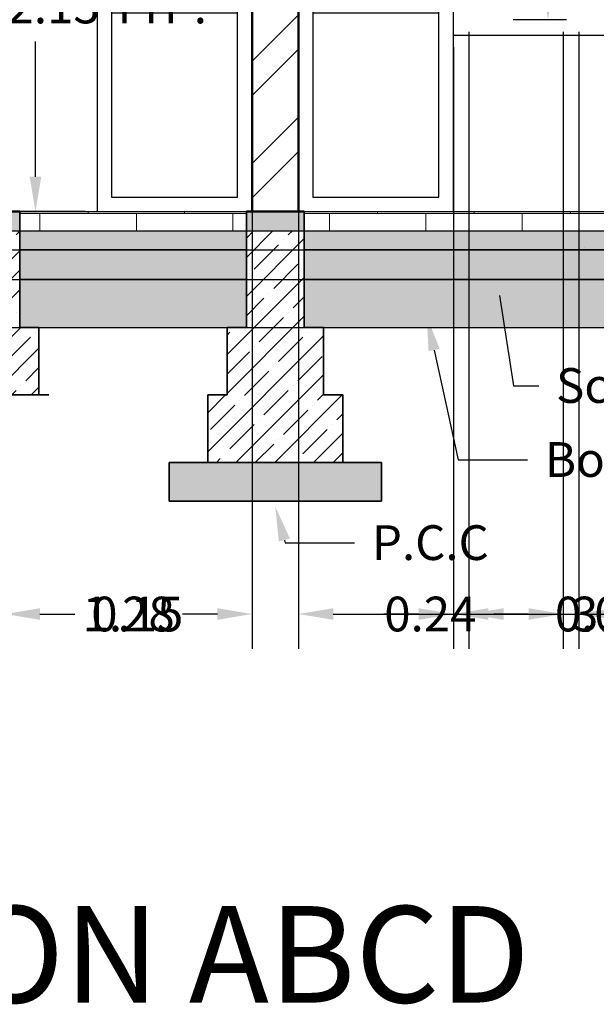
# Model space of a CAD drawing. Units: metres. Extents: x 22.1 to 34.4, y 4.4 to 12.4.
# Tile 2 of 8: x 26.6 to 29.6, y 4.4 to 9.5. Entities that reach past the tile are written whole.
import ezdxf
from ezdxf import colors
from ezdxf.entities.mleader import LeaderData, LeaderLine
from ezdxf.math import Vec2, Vec3

# ---------------------------------------------------------------- set-up
doc = ezdxf.new("R2010")
doc.units = ezdxf.units.M
doc.header["$MEASUREMENT"] = 0
for name, color, linetype, lineweight in [('A-ANNO-DIMS', 2, 'Continuous', 18), ('A-ANNO-TEXT', 7, 'Continuous', 18), ('A-DOOR', 4, 'Continuous', 25), ('A-FLOR', 3, 'Continuous', 25), ('A-FLOR-PATT', 252, 'Continuous', 13), ('A-GLAZ', 4, 'Continuous', 25), ('A-WALL', 7, 'Continuous', 50), ('A-WALL-PATT', 8, 'Continuous', 18), ('S-FNDN', 1, 'Continuous', 35), ('S-FNDN-PATT', 8, 'Continuous', 13), ('S-SLAB-PATT', 8, 'Continuous', 13)]:
    doc.layers.add(name, color=color, linetype=linetype, lineweight=lineweight)
doc.styles.get("Standard").update_dxf_attribs({"font": 'arial.ttf'})
doc.dimstyles.get("Standard").update_dxf_attribs({"dimtxt": 0.18, "dimasz": 0.18, "dimexe": 0.18, "dimexo": 0.0625, "dimgap": 0.09, "dimtad": 0, "dimtih": 1, "dimtoh": 1, "dimzin": 0, "dimdsep": 46, "dimtxsty": 'Standard', "dimcen": 0.09, "dimadec": 0, "dimazin": 0, "dimtfac": 1, "dimtofl": 0, "dimtmove": 0, "dimatfit": 3, "dimfxl": 1, "dimtolj": 1, "dimtzin": 0, "dimarcsym": 0})

# ---------------------------------------------------------------- blocks, each defined once
blk = doc.blocks.new('DOOR-800')
for p, q in [((26.4206, 10.6399), (25.6173, 10.6399)), ((25.6173, 10.6399), (25.6173, 8.5099)), ((26.4206, 8.5099), (26.4206, 10.6399)), ((25.6923, 10.5649), (25.6923, 8.5849)), ((26.3456, 10.5649), (25.6923, 10.5649)), ((26.3456, 8.5849), (26.3456, 10.5649)), ((25.6923, 9.6099), (26.3456, 9.6099)), ((25.6923, 9.5399), (26.3456, 9.5399)), ((25.6923, 8.5849), (26.3456, 8.5849)), ((25.6173, 8.5099), (26.4206, 8.5099))]:
    blk.add_line(p, q)
blk = doc.blocks.new('*D16')
at = {"layer": 'A-ANNO-DIMS', "color": 0, "lineweight": -2, "transparency": 16777216}
for p, q in [((26.9843, 10.6399), (26.5473, 10.6399)), ((26.7273, 10.4599), (26.7273, 9.7581)), ((26.7273, 8.6899), (26.7273, 9.3917)), ((26.9843, 8.5099), (26.5473, 8.5099))]:
    blk.add_line(p, q, dxfattribs=at)
at = {"layer": 'A-ANNO-DIMS', "color": 0, "transparency": 16777216}
for points in [[(26.6973, 10.4599), (26.7573, 10.4599), (26.7273, 10.6399)], [(26.6973, 8.6899), (26.7573, 8.6899), (26.7273, 8.5099)]]:
    blk.add_solid(points, dxfattribs=at)
at = {"layer": 'Defpoints', "color": 0, "transparency": 16777216}
for p in [(26.7273, 10.6399), (27.0468, 10.6399), (27.0468, 8.5099)]:
    blk.add_point(p, dxfattribs=at)
at = {"layer": 'A-ANNO-DIMS', "color": 0, "transparency": 16777216, "insert": (26.7273, 9.5749), "char_height": 0.18, "attachment_point": 5}
blk.add_mtext('\\A1;DOOR 2.13 TYP.', dxfattribs=at)
blk = doc.blocks.new('*D20')
at = {"layer": 'A-ANNO-DIMS', "color": 0, "lineweight": -2, "transparency": 16777216}
for p, q in [((29.4798, 10.5649), (29.2032, 10.5649)), ((29.3832, 10.3849), (29.3832, 10.2176)), ((29.3832, 9.6839), (29.3832, 9.8512)), ((29.4798, 9.5039), (29.2032, 9.5039))]:
    blk.add_line(p, q, dxfattribs=at)
at = {"layer": 'A-ANNO-DIMS', "color": 0, "transparency": 16777216}
for points in [[(29.3532, 10.3849), (29.4132, 10.3849), (29.3832, 10.5649)], [(29.3532, 9.6839), (29.4132, 9.6839), (29.3832, 9.5039)]]:
    blk.add_solid(points, dxfattribs=at)
at = {"layer": 'Defpoints', "color": 0, "transparency": 16777216}
for p in [(29.3832, 10.5649), (29.5423, 10.5649), (29.5423, 9.5039)]:
    blk.add_point(p, dxfattribs=at)
at = {"layer": 'A-ANNO-DIMS', "color": 0, "transparency": 16777216, "insert": (29.3832, 10.0344), "char_height": 0.18, "attachment_point": 5}
blk.add_mtext('\\A1;WINDOW PANE 530 1.06 TYP.', dxfattribs=at)
blk = doc.blocks.new('*D23')
at = {"layer": 'A-ANNO-DIMS', "color": 0, "lineweight": -2, "transparency": 16777216}
for p, q in [((28.0901, 11.4474), (28.0901, 6.2449)), ((31.5381, 11.4474), (31.5381, 6.2449)), ((28.2701, 6.4249), (29.4202, 6.4249)), ((31.3581, 6.4249), (30.2079, 6.4249))]:
    blk.add_line(p, q, dxfattribs=at)
at = {"layer": 'A-ANNO-DIMS', "color": 0, "transparency": 16777216}
for points in [[(28.2701, 6.4549), (28.2701, 6.3949), (28.0901, 6.4249)], [(31.3581, 6.4549), (31.3581, 6.3949), (31.5381, 6.4249)]]:
    blk.add_solid(points, dxfattribs=at)
at = {"layer": 'Defpoints', "color": 0, "transparency": 16777216}
for p in [(28.0901, 11.5099), (31.5381, 11.5099), (31.5381, 6.4249)]:
    blk.add_point(p, dxfattribs=at)
at = {"layer": 'A-ANNO-DIMS', "color": 0, "transparency": 16777216, "insert": (29.8141, 6.4249), "char_height": 0.18, "attachment_point": 5}
blk.add_mtext('\\A1;3.448', dxfattribs=at)
blk = doc.blocks.new('*D26')
at = {"layer": 'A-ANNO-DIMS', "color": 0, "lineweight": -2, "transparency": 16777216}
for p, q in [((27.8501, 11.4474), (27.8501, 6.2449)), ((28.0901, 11.4474), (28.0901, 6.2449)), ((27.6701, 6.4249), (27.4901, 6.4249)), ((28.2701, 6.4249), (28.4501, 6.4249))]:
    blk.add_line(p, q, dxfattribs=at)
at = {"layer": 'A-ANNO-DIMS', "color": 0, "transparency": 16777216}
for points in [[(27.6701, 6.4549), (27.6701, 6.3949), (27.8501, 6.4249)], [(28.2701, 6.4549), (28.2701, 6.3949), (28.0901, 6.4249)]]:
    blk.add_solid(points, dxfattribs=at)
at = {"layer": 'Defpoints', "color": 0, "transparency": 16777216}
for p in [(27.8501, 11.5099), (28.0901, 11.5099), (28.0901, 6.4249)]:
    blk.add_point(p, dxfattribs=at)
at = {"layer": 'A-ANNO-DIMS', "color": 0, "transparency": 16777216, "insert": (28.7735, 6.4249), "char_height": 0.18, "attachment_point": 5}
blk.add_mtext('\\A1;0.24', dxfattribs=at)
blk = doc.blocks.new('*D31')
at = {"layer": 'A-ANNO-DIMS', "color": 0, "lineweight": -2, "transparency": 16777216}
for p, q in [((26.4206, 8.4474), (26.4206, 6.2449)), ((26.5706, 8.4474), (26.5706, 6.2449)), ((26.2406, 6.4249), (26.0606, 6.4249)), ((26.7506, 6.4249), (26.9306, 6.4249))]:
    blk.add_line(p, q, dxfattribs=at)
at = {"layer": 'A-ANNO-DIMS', "color": 0, "transparency": 16777216}
for points in [[(26.2406, 6.4549), (26.2406, 6.3949), (26.4206, 6.4249)], [(26.7506, 6.4549), (26.7506, 6.3949), (26.5706, 6.4249)]]:
    blk.add_solid(points, dxfattribs=at)
at = {"layer": 'Defpoints', "color": 0, "transparency": 16777216}
for p in [(26.4206, 8.5099), (26.5706, 8.5099), (26.5706, 6.4249)]:
    blk.add_point(p, dxfattribs=at)
at = {"layer": 'A-ANNO-DIMS', "color": 0, "transparency": 16777216, "insert": (27.255, 6.4249), "char_height": 0.18, "attachment_point": 5}
blk.add_mtext('\\A1;0.15', dxfattribs=at)
blk = doc.blocks.new('*D32')
at = {"layer": 'A-ANNO-DIMS', "color": 0, "lineweight": -2, "transparency": 16777216}
for p, q in [((26.5706, 8.4474), (26.5706, 6.2449)), ((27.8501, 8.4474), (27.8501, 6.2449)), ((26.7506, 6.4249), (26.8948, 6.4249)), ((27.6701, 6.4249), (27.5258, 6.4249))]:
    blk.add_line(p, q, dxfattribs=at)
at = {"layer": 'A-ANNO-DIMS', "color": 0, "transparency": 16777216}
for points in [[(26.7506, 6.4549), (26.7506, 6.3949), (26.5706, 6.4249)], [(27.6701, 6.4549), (27.6701, 6.3949), (27.8501, 6.4249)]]:
    blk.add_solid(points, dxfattribs=at)
at = {"layer": 'Defpoints', "color": 0, "transparency": 16777216}
for p in [(26.5706, 8.5099), (27.8501, 8.5099), (27.8501, 6.4249)]:
    blk.add_point(p, dxfattribs=at)
at = {"layer": 'A-ANNO-DIMS', "color": 0, "transparency": 16777216, "insert": (27.2103, 6.4249), "char_height": 0.18, "attachment_point": 5}
blk.add_mtext('\\A1;1.28', dxfattribs=at)
blk = doc.blocks.new('*D34')
at = {"layer": 'A-ANNO-DIMS', "color": 0, "lineweight": -2, "transparency": 16777216}
for p, q in [((28.8933, 9.3614), (28.8933, 6.2449)), ((31.3293, 9.3614), (31.3293, 6.2449)), ((29.0733, 6.4249), (29.7162, 6.4249)), ((31.1493, 6.4249), (30.5065, 6.4249))]:
    blk.add_line(p, q, dxfattribs=at)
at = {"layer": 'A-ANNO-DIMS', "color": 0, "transparency": 16777216}
for points in [[(29.0733, 6.4549), (29.0733, 6.3949), (28.8933, 6.4249)], [(31.1493, 6.4549), (31.1493, 6.3949), (31.3293, 6.4249)]]:
    blk.add_solid(points, dxfattribs=at)
at = {"layer": 'Defpoints', "color": 0, "transparency": 16777216}
for p in [(28.8933, 9.4239), (31.3293, 9.4239), (31.3293, 6.4249)]:
    blk.add_point(p, dxfattribs=at)
at = {"layer": 'A-ANNO-DIMS', "color": 0, "transparency": 16777216, "insert": (30.1113, 6.4249), "char_height": 0.18, "attachment_point": 5}
blk.add_mtext('\\A1;2.436', dxfattribs=at)
blk = doc.blocks.new('*D35')
at = {"layer": 'A-ANNO-DIMS', "color": 0, "lineweight": -2, "transparency": 16777216}
for p, q in [((28.9733, 9.4414), (28.9733, 6.2449)), ((28.8933, 9.3614), (28.8933, 6.2449)), ((28.7133, 6.4249), (28.5333, 6.4249)), ((29.1533, 6.4249), (29.3333, 6.4249))]:
    blk.add_line(p, q, dxfattribs=at)
at = {"layer": 'A-ANNO-DIMS', "color": 0, "transparency": 16777216}
for points in [[(28.7133, 6.4549), (28.7133, 6.3949), (28.8933, 6.4249)], [(29.1533, 6.4549), (29.1533, 6.3949), (28.9733, 6.4249)]]:
    blk.add_solid(points, dxfattribs=at)
at = {"layer": 'Defpoints', "color": 0, "transparency": 16777216}
for p in [(28.9733, 9.5039), (28.8933, 9.4239), (28.9733, 6.4249)]:
    blk.add_point(p, dxfattribs=at)
at = {"layer": 'A-ANNO-DIMS', "color": 0, "transparency": 16777216, "insert": (29.6573, 6.4249), "char_height": 0.18, "attachment_point": 5}
blk.add_mtext('\\A1;0.08', dxfattribs=at)
blk = doc.blocks.new('*D36')
at = {"layer": 'A-ANNO-DIMS', "color": 0, "lineweight": -2, "transparency": 16777216}
for p, q in [((29.4623, 9.4414), (29.4623, 6.2449)), ((29.5423, 9.4414), (29.5423, 6.2449)), ((29.2823, 6.4249), (29.1023, 6.4249)), ((29.7223, 6.4249), (29.9023, 6.4249))]:
    blk.add_line(p, q, dxfattribs=at)
at = {"layer": 'A-ANNO-DIMS', "color": 0, "transparency": 16777216}
for points in [[(29.2823, 6.4549), (29.2823, 6.3949), (29.4623, 6.4249)], [(29.7223, 6.4549), (29.7223, 6.3949), (29.5423, 6.4249)]]:
    blk.add_solid(points, dxfattribs=at)
at = {"layer": 'Defpoints', "color": 0, "transparency": 16777216}
for p in [(29.4623, 9.5039), (29.5423, 9.5039), (29.5423, 6.4249)]:
    blk.add_point(p, dxfattribs=at)
at = {"layer": 'A-ANNO-DIMS', "color": 0, "transparency": 16777216, "insert": (30.2263, 6.4249), "char_height": 0.18, "attachment_point": 5}
blk.add_mtext('\\A1;0.08', dxfattribs=at)
blk = doc.blocks.new('*D44')
at = {"layer": 'A-ANNO-DIMS', "color": 0, "lineweight": -2, "transparency": 16777216}
for p, q in [((33.6737, 8.6899), (33.6737, 8.8699)), ((24.8474, 8.5099), (33.8537, 8.5099)), ((24.5474, 8.4099), (33.8537, 8.4099)), ((33.6737, 8.2299), (33.6737, 8.0499)), ((33.6737, 8.0499), (33.4937, 8.0499))]:
    blk.add_line(p, q, dxfattribs=at)
at = {"layer": 'A-ANNO-DIMS', "color": 0, "transparency": 16777216}
for points in [[(33.6437, 8.6899), (33.7037, 8.6899), (33.6737, 8.5099)], [(33.6437, 8.2299), (33.7037, 8.2299), (33.6737, 8.4099)]]:
    blk.add_solid(points, dxfattribs=at)
at = {"layer": 'Defpoints', "color": 0, "transparency": 16777216}
for p in [(24.7849, 8.5099), (24.4849, 8.4099), (33.6737, 8.4099)]:
    blk.add_point(p, dxfattribs=at)
at = {"layer": 'A-ANNO-DIMS', "color": 0, "transparency": 16777216, "insert": (33.1702, 8.0499), "char_height": 0.18, "attachment_point": 5}
blk.add_mtext('\\A1;0.10', dxfattribs=at)
blk = doc.blocks.new('*D45')
at = {"layer": 'A-ANNO-DIMS', "color": 0, "lineweight": -2, "transparency": 16777216}
for p, q in [((33.6737, 8.5899), (33.6737, 8.7699)), ((24.5474, 8.4099), (33.8537, 8.4099)), ((24.8474, 8.3119), (33.8537, 8.3119)), ((33.6737, 8.1319), (33.6737, 7.9519)), ((33.6737, 7.9519), (33.4937, 7.9519))]:
    blk.add_line(p, q, dxfattribs=at)
at = {"layer": 'A-ANNO-DIMS', "color": 0, "transparency": 16777216}
for points in [[(33.6437, 8.5899), (33.7037, 8.5899), (33.6737, 8.4099)], [(33.6437, 8.1319), (33.7037, 8.1319), (33.6737, 8.3119)]]:
    blk.add_solid(points, dxfattribs=at)
at = {"layer": 'Defpoints', "color": 0, "transparency": 16777216}
for p in [(24.4849, 8.4099), (24.7849, 8.3119), (33.6737, 8.3119)]:
    blk.add_point(p, dxfattribs=at)
at = {"layer": 'A-ANNO-DIMS', "color": 0, "transparency": 16777216, "insert": (33.0998, 7.9519), "char_height": 0.18, "attachment_point": 5}
blk.add_mtext('\\A1;0.098', dxfattribs=at)
blk = doc.blocks.new('*D46')
at = {"layer": 'A-ANNO-DIMS', "color": 0, "lineweight": -2, "transparency": 16777216}
for p, q in [((33.6737, 8.4919), (33.6737, 8.6719)), ((24.8474, 8.3119), (33.8537, 8.3119)), ((24.8474, 8.1578), (33.8537, 8.1578)), ((33.6737, 7.9778), (33.6737, 7.7978)), ((33.6737, 7.7978), (33.4937, 7.7978))]:
    blk.add_line(p, q, dxfattribs=at)
at = {"layer": 'A-ANNO-DIMS', "color": 0, "transparency": 16777216}
for points in [[(33.6437, 8.4919), (33.7037, 8.4919), (33.6737, 8.3119)], [(33.6437, 7.9778), (33.7037, 7.9778), (33.6737, 8.1578)]]:
    blk.add_solid(points, dxfattribs=at)
at = {"layer": 'Defpoints', "color": 0, "transparency": 16777216}
for p in [(24.7849, 8.3119), (24.7849, 8.1578), (33.6737, 8.1578)]:
    blk.add_point(p, dxfattribs=at)
at = {"layer": 'A-ANNO-DIMS', "color": 0, "transparency": 16777216, "insert": (33.1692, 7.7978), "char_height": 0.18, "attachment_point": 5}
blk.add_mtext('\\A1;0.15', dxfattribs=at)
blk = doc.blocks.new('*D47')
at = {"layer": 'A-ANNO-DIMS', "color": 0, "lineweight": -2, "transparency": 16777216}
for p, q in [((33.6737, 8.3378), (33.6737, 8.5178)), ((24.8474, 8.1578), (33.8537, 8.1578)), ((24.8474, 7.9099), (33.8537, 7.9099)), ((33.6737, 7.7299), (33.6737, 7.5499)), ((33.6737, 7.5499), (33.4937, 7.5499))]:
    blk.add_line(p, q, dxfattribs=at)
at = {"layer": 'A-ANNO-DIMS', "color": 0, "transparency": 16777216}
for points in [[(33.6437, 8.3378), (33.7037, 8.3378), (33.6737, 8.1578)], [(33.6437, 7.7299), (33.7037, 7.7299), (33.6737, 7.9099)]]:
    blk.add_solid(points, dxfattribs=at)
at = {"layer": 'Defpoints', "color": 0, "transparency": 16777216}
for p in [(24.7849, 8.1578), (24.7849, 7.9099), (33.6737, 7.9099)]:
    blk.add_point(p, dxfattribs=at)
at = {"layer": 'A-ANNO-DIMS', "color": 0, "transparency": 16777216, "insert": (33.1692, 7.5499), "char_height": 0.18, "attachment_point": 5}
blk.add_mtext('\\A1;0.25', dxfattribs=at)

msp = doc.modelspace()

# ---------------------------------------------------------------- hatches: boundary and pattern name
at = {"layer": 'A-FLOR-PATT'}
h = msp.add_hatch(dxfattribs=at)
h.set_pattern_fill('BRICK', color=256)
h.paths.add_polyline_path([(31.5081, 8.5099), (28.1201, 8.5099), (28.1201, 8.4099), (31.5081, 8.4099)])
h.paths.add_polyline_path([(27.8201, 8.5099), (27.0468, 8.5099), (26.6456, 8.5099), (26.6456, 8.4099), (27.8201, 8.4099)])
h.paths.add_polyline_path([(26.3456, 8.5099), (25.6173, 8.5099), (24.7849, 8.5099), (24.7849, 8.4099), (26.3456, 8.4099)])
h = msp.add_hatch(dxfattribs=at)
h.set_pattern_fill('AR-SAND', color=256, scale=0.57)
h.paths.add_polyline_path([(26.3456, 8.4099), (24.7849, 8.4099), (24.7849, 8.3119), (26.3456, 8.3119)])
h.paths.add_polyline_path([(27.8201, 8.4099), (26.6456, 8.4099), (26.6456, 8.3119), (27.8201, 8.3119)])
h.paths.add_polyline_path([(31.5081, 8.4099), (28.1201, 8.4099), (28.1201, 8.3119), (31.5081, 8.3119)])
h = msp.add_hatch(dxfattribs=at)
h.set_pattern_fill('AR-SAND', color=256, scale=0.57)
h.paths.add_polyline_path([(31.5081, 8.4099), (28.1201, 8.4099), (28.1201, 8.3119), (31.5081, 8.3119)])
h.paths.add_polyline_path([(27.8201, 8.4099), (26.6456, 8.4099), (26.6456, 8.3119), (27.8201, 8.3119)])
h.paths.add_polyline_path([(26.3456, 8.4099), (24.7849, 8.4099), (24.7849, 8.3119), (26.3456, 8.3119)])
h = msp.add_hatch(dxfattribs=at)
h.set_pattern_fill('AR-SAND', color=256, scale=0.04)
h.paths.add_polyline_path([(26.3456, 8.4099), (24.7849, 8.4099), (24.7849, 8.3119), (26.3456, 8.3119)])
h.paths.add_polyline_path([(27.8201, 8.4099), (26.6456, 8.4099), (26.6456, 8.3119), (27.8201, 8.3119)])
h.paths.add_polyline_path([(31.5081, 8.4099), (28.1201, 8.4099), (28.1201, 8.3119), (31.5081, 8.3119)])
h = msp.add_hatch(dxfattribs=at)
h.set_pattern_fill('GRAVEL', color=256, scale=0.18)
h.set_pattern_definition([(228.012788, (0.1296, 0.18), (-1.44, -1.62), [0.0242165, -2.39743585]), (184.96974, (0.1134, 0.162), (2.16, 0.18), [0.0415562, -4.1140665]), (132.510447, (0.072, 0.1584), (1.8, -1.98), [0.0293018, -2.9008859]), (267.27369, (0.0018, 0.1134), (0.18, 3.6), [0.0378428, -3.74644045]), (292.833654, (0, 0.0756), (-0.9, 2.16), [0.0371079, -3.6736872]), (357.27369, (0.0144, 0.0414), (-3.6, 0.18), [0.0378428, -3.74644045]), (37.69424, (0.0522, 0.0396), (-2.34, -1.8), [0.0500452, -4.9544727]), (72.255328, (0.0918, 0.0702), (1.26, 3.96), [0.0472478, -4.6775379]), (121.429566, (0.1062, 0.1152), (-1.44, 2.34), [0.037971, -3.7591332]), (175.23636, (0.0864, 0.1476), (1.98, -0.18), [0.0433498, -2.1241373]), (222.397438, (0.0432, 0.1512), (-2.16, -1.98), [0.0560606, -5.5500075]), (138.814075, (0.18, 0.1116), (-1.26, 1.08), [0.0191342, -1.8942921]), (171.469234, (0.1656, 0.1242), (2.34, -0.36), [0.0364027, -3.60387205]), (225, (0.1296, 0.1296), (0, -0.18), [0.0254558, -0.2291027]), (203.19859, (0.117, 0.1512), (0.9, 0.36), [0.0137084, -1.3571307]), (291.80141, (0.1044, 0.1458), (-0.18, 0.54), [0.0193865, -0.9499431]), (30.96376, (0.1116, 0.1278), (0.54, 0.36), [0.0314872, -1.0180841]), (161.56505, (0.1386, 0.144), (0.36, -0.18), [0.0227684, -0.5464416]), (16.38954, (0, 0.1458), (1.8, 0.54), [0.031896, -3.1577121]), (70.346176, (0.0306, 0.1548), (-0.72, -1.98), [0.026759, -2.6491334]), (293.19859, (0.1386, 0.18), (-0.36, 0.9), [0.0274167, -1.3434225]), (343.61046, (0.1494, 0.1548), (-1.8, 0.54), [0.031896, -3.1577121]), (339.443955, (0, 0.0342), (-0.9, 0.36), [0.0307584, -1.5071623]), (294.77514, (0.0288, 0.0234), (-0.9, 1.98), [0.025772, -2.55143575]), (66.80141, (0.1404, 0), (0.36, 0.9), [0.0274167, -1.3434225]), (17.354025, (0.1512, 0.0252), (-2.34, -0.72), [0.0301736, -2.98717625]), (69.443955, (0.0522, 0), (-0.36, -0.9), [0.0153792, -1.5225415]), (101.30993, (0.1296, 0), (-0.18, 0.72), [0.0091782, -0.9086453]), (165.96376, (0.1278, 0.009), (0.54, -0.18), [0.0371079, -0.7050511]), (186.009006, (0.0918, 0.018), (1.8, 0.18), [0.034389, -3.4045062]), (303.69007, (0.1116, 0.1116), (-0.18, 0.36), [0.02596, -0.6230393]), (353.157227, (0.126, 0.09), (3.06, -0.36), [0.0453229, -4.4869613]), (60.945396, (0.171, 0.0846), (-0.72, -1.26), [0.0185321, -1.8346813]), (90, (0.18, 0.1008), (-0.18, 0.18), [0.0108, -0.1692]), (120.256437, (0.0882, 0.0234), (0.72, -1.26), [0.0250063, -2.4756336]), (48.012788, (0.0756, 0.045), (1.44, 1.62), [0.048433, -2.3732194]), (0, (0.108, 0.081), (0.18, 0.18), [0.0468, -0.1332]), (325.304846, (0.1548, 0.081), (1.8, -1.26), [0.0284605, -2.8175894]), (254.0546, (0.1782, 0.0648), (-0.18, -0.72), [0.0262084, -1.2842114]), (207.645975, (0.171, 0.0396), (-3.42, -1.8), [0.0426717, -4.22450535]), (175.42608, (0.1332, 0.0198), (-2.34, 0.18), [0.0451438, -4.4692332])])
h.paths.add_polyline_path([(26.3456, 8.1578), (24.7849, 8.1578), (24.7849, 7.9099), (24.8849, 7.9099), (26.3456, 7.9099)])
h.paths.add_polyline_path([(27.8201, 8.1578), (26.6456, 8.1578), (26.6456, 7.9099), (26.7456, 7.9099), (27.8201, 7.9099)])
h.paths.add_polyline_path([(31.5081, 8.1578), (28.1201, 8.1578), (28.1201, 7.9099), (31.4081, 7.9099), (31.5081, 7.9099)])
at = {"layer": 'A-WALL-PATT'}
h = msp.add_hatch(dxfattribs=at)
h.set_pattern_fill('ANSI32', color=256)
h.paths.add_polyline_path([(24.7549, 11.5099), (24.5149, 11.5099), (24.5149, 11.1399), (24.7549, 11.1399)])
h.paths.add_polyline_path([(24.7549, 10.6399), (24.5149, 10.6399), (24.5149, 8.5099), (24.6349, 8.5099), (24.7549, 8.5099)])
h.paths.add_polyline_path([(26.5706, 11.5099), (26.4206, 11.5099), (26.4206, 8.5099), (26.5706, 8.5099)])
h.paths.add_polyline_path([(28.0901, 10.6399), (28.0901, 11.5099), (27.8501, 11.5099), (27.8501, 8.5099), (28.0901, 8.5099)])
h.paths.add_polyline_path([(31.7781, 11.5099), (31.5381, 11.5099), (31.5381, 8.5099), (31.6581, 8.5099), (31.7781, 8.5099)])
at = {"layer": 'S-FNDN-PATT'}
h = msp.add_hatch(dxfattribs=at)
h.set_pattern_fill('ANSI35', color=256, scale=0.57)
h.paths.add_polyline_path([(24.3849, 7.5599), (24.2849, 7.5599), (24.2849, 7.2099), (24.9849, 7.2099), (24.9849, 7.5599), (24.8849, 7.5599), (24.8849, 7.9099), (24.7849, 7.9099), (24.7849, 8.4099), (24.4849, 8.4099), (24.4849, 7.9099), (24.3849, 7.9099)])
h.paths.add_polyline_path([(27.7201, 7.5599), (27.6201, 7.5599), (27.6201, 7.2099), (28.3201, 7.2099), (28.3201, 7.5599), (28.2201, 7.5599), (28.2201, 7.9099), (28.1201, 7.9099), (28.1201, 8.4099), (27.8201, 8.4099), (27.8201, 7.9099), (27.7201, 7.9099)])
h.paths.add_polyline_path([(26.7456, 7.9099), (26.6456, 7.9099), (26.6456, 8.4099), (26.3456, 8.4099), (26.3456, 7.9099), (26.2456, 7.9099), (26.2456, 7.5599), (26.4616, 7.5599), (26.4616, 7.6127), (26.4825, 7.5003), (26.4825, 7.5599), (26.7456, 7.5599)])
h.paths.add_polyline_path([(31.8581, 7.5599), (31.8581, 7.9099), (31.8081, 7.9099), (31.8081, 8.4099), (31.5081, 8.4099), (31.5081, 7.9099), (31.4581, 7.9099), (31.4581, 7.5599), (31.3581, 7.5599), (31.3581, 7.2099), (31.9581, 7.2099), (31.9581, 7.5599)])
at = {"layer": 'S-SLAB-PATT'}
h = msp.add_hatch(dxfattribs=at)
h.set_pattern_fill('AR-CONC', color=256, scale=0.04)
h.set_pattern_definition([(50, (0, 0), (0.286904, -0.0251009), [0.03, -0.33]), (355, (0, 0), (-0.0555005, 0.3008769), [0.024, -0.264]), (100.4514, (0.0239, -0.0021), (0.2314035, 0.275776), [0.025496, -0.2804568]), (46.1842, (0, 0.08), (0.4268965, -0.0662077), [0.045, -0.495]), (96.6356, (0.03557, 0.0745), (0.373865, 0.3896474), [0.038244, -0.4206855]), (351.1842, (0, 0.08), (0.373865, 0.3896474), [0.036, -0.396]), (21, (0.04, 0.06), (0.2387628, -0.1610476), [0.03, -0.33]), (326, (0.04, 0.06), (0.0973261, 0.29006), [0.024, -0.264]), (71.4514, (0.0599, 0.04658), (0.336089, 0.1290125), [0.025496, -0.2804568]), (37.5, (0, 0), (0.00486394, 0.13315754), [0, -0.2608, 0, -0.268, 0, -0.265]), (7.5, (0, 0), (0.1052278, 0.1577647), [0, -0.1528, 0, -0.2548, 0, -0.101]), (327.5, (-0.0892, 0), (0.21352897, -0.00902195), [0, -0.1, 0, -0.312, 0, -0.414]), (317.5, (-0.1292, 0), (0.2332745, 0.040042), [0, -0.13, 0, -0.2072, 0, -0.294])])
h.paths.add_polyline_path([(31.9781, 11.6599), (24.3149, 11.6599), (24.3149, 11.5099), (24.5149, 11.5099), (31.7781, 11.5099), (31.9781, 11.5099)])
h.paths.add_polyline_path([(25.1849, 7.2099), (24.9849, 7.2099), (24.0849, 7.2099), (24.0849, 7.0099), (25.1849, 7.0099)])
h.paths.add_polyline_path([(32.2081, 7.2099), (32.0081, 7.2099), (31.1081, 7.2099), (31.1081, 7.0099), (32.2081, 7.0099)])
h.paths.add_polyline_path([(28.5201, 7.2099), (28.3201, 7.2099), (27.4201, 7.2099), (27.4201, 7.0099), (28.5201, 7.0099)])
h.paths.add_polyline_path([(24.7849, 8.5099), (24.6349, 8.5099), (24.5149, 8.5099), (24.4849, 8.5099), (24.4849, 8.4099), (24.7849, 8.4099)])
h.paths.add_polyline_path([(26.6456, 8.5099), (26.3456, 8.5099), (26.3456, 8.4099), (26.6456, 8.4099)])
h.paths.add_polyline_path([(28.1201, 8.5099), (28.0901, 8.5099), (27.8201, 8.5099), (27.8201, 8.4099), (28.1201, 8.4099)])
h.paths.add_polyline_path([(31.8081, 8.5099), (31.6581, 8.5099), (31.5381, 8.5099), (31.5081, 8.5099), (31.5081, 8.4099), (31.8081, 8.4099)])
h.paths.add_polyline_path([(26.3456, 8.3119), (24.7849, 8.3119), (24.7849, 8.1578), (26.3456, 8.1578)])
h.paths.add_polyline_path([(27.8201, 8.3119), (26.6456, 8.3119), (26.6456, 8.1578), (27.8201, 8.1578)])
h.paths.add_polyline_path([(31.5081, 8.3119), (28.1201, 8.3119), (28.1201, 8.1578), (31.5081, 8.1578)])

# ---------------------------------------------------------------- linework, layer by layer
at = {"layer": 'A-FLOR'}
for p, q in [((24.7849, 8.5099), (31.5081, 8.5099)), ((26.6456, 8.4099), (28.1201, 8.4099)), ((28.1201, 8.4099), (31.8081, 8.4099)), ((27.8201, 8.3119), (26.6456, 8.3119)), ((31.5081, 8.3119), (28.1201, 8.3119)), ((27.8201, 8.1578), (26.6456, 8.1578)), ((31.5081, 8.1578), (28.1201, 8.1578)), ((26.6456, 7.9099), (27.8201, 7.9099)), ((28.1201, 7.9099), (31.4081, 7.9099))]:
    msp.add_line(p, q, dxfattribs=at)
at = {"layer": 'A-GLAZ'}
msp.add_line((28.8933, 9.4239), (31.3293, 9.4239), dxfattribs=at)
at = {"layer": 'A-WALL'}
for p, q in [((27.8501, 8.5099), (27.8501, 11.5099)), ((28.0901, 8.5099), (28.0901, 11.5099)), ((26.3456, 8.5099), (26.6456, 8.5099)), ((27.8201, 8.5099), (27.9701, 8.5099)), ((27.9701, 8.5099), (27.8501, 8.5099)), ((28.1201, 8.5099), (27.9701, 8.5099)), ((27.9701, 8.5099), (28.0901, 8.5099))]:
    msp.add_line(p, q, dxfattribs=at)
at = {"layer": 'S-FNDN'}
for p, q in [((26.6456, 7.9099), (26.6456, 8.5099)), ((27.8201, 7.9099), (27.8201, 8.5099)), ((28.1201, 7.9099), (28.1201, 8.5099)), ((26.6456, 7.9099), (26.7456, 7.9099)), ((26.7456, 7.5599), (26.7456, 7.9099)), ((27.7201, 7.5599), (27.7201, 7.9099)), ((27.7201, 7.9099), (27.8201, 7.9099)), ((28.2201, 7.9099), (28.1201, 7.9099)), ((28.2201, 7.5599), (28.2201, 7.9099)), ((26.4825, 7.5599), (26.7961, 7.5599)), ((27.6201, 7.2099), (27.6201, 7.5599)), ((27.6201, 7.5599), (27.7201, 7.5599)), ((28.3201, 7.5599), (28.2201, 7.5599)), ((28.3201, 7.2099), (28.3201, 7.5599)), ((27.4201, 7.0099), (27.4201, 7.2099)), ((27.4201, 7.2099), (28.3201, 7.2099)), ((28.5201, 7.2099), (28.3201, 7.2099)), ((28.5201, 7.0099), (28.5201, 7.2099)), ((27.4201, 7.0099), (28.5201, 7.0099))]:
    msp.add_line(p, q, dxfattribs=at)

# ---------------------------------------------------------------- block references
at = {"layer": 'A-DOOR'}
for p in [(1.4295, 0), (2.4728, 0)]:
    msp.add_blockref('DOOR-800', p, dxfattribs=at)

# ---------------------------------------------------------------- texts
at = {"layer": 'A-ANNO-TEXT', "insert": (24.5182, 4.9119), "char_height": 0.5, "attachment_point": 1}
msp.add_mtext_dynamic_manual_height_columns('SECTION ABCD', width=6.025695, gutter_width=0.858, heights=[0], dxfattribs=at)

# ---------------------------------------------------------------- dimensions: what is measured, and where the dimension line sits
at = {"layer": 'A-ANNO-DIMS'}
for base, p1, p2, override, picture, middle in [((28.0901, 6.4249), (27.8501, 11.5099), (28.0901, 11.5099), {"dimdec": 2, "dimlfac": 1, "dimrnd": 0, "dimzin": 0, "dimdsep": 46, "dimlunit": 2}, '*D26', (28.7735, 6.4249)), ((31.5381, 6.4249), (28.0901, 11.5099), (31.5381, 11.5099), {"dimdec": 3, "dimlfac": 1, "dimrnd": 0, "dimzin": 0, "dimdsep": 46, "dimlunit": 2}, '*D23', (29.8141, 6.4249)), ((28.9733, 6.4249), (28.8933, 9.4239), (28.9733, 9.5039), {"dimdec": 2, "dimlfac": 1, "dimrnd": 0, "dimzin": 0, "dimdsep": 46, "dimlunit": 2}, '*D35', (29.6573, 6.4249)), ((29.5423, 6.4249), (29.4623, 9.5039), (29.5423, 9.5039), {"dimdec": 2, "dimlfac": 1, "dimrnd": 0, "dimzin": 0, "dimdsep": 46, "dimlunit": 2}, '*D36', (30.2263, 6.4249)), ((31.3293, 6.4249), (28.8933, 9.4239), (31.3293, 9.4239), {"dimdec": 3, "dimlfac": 1, "dimrnd": 0, "dimzin": 0, "dimdsep": 46, "dimlunit": 2}, '*D34', (30.1113, 6.4249)), ((26.5706, 6.4249), (26.4206, 8.5099), (26.5706, 8.5099), {"dimdec": 2, "dimlfac": 1, "dimrnd": 0, "dimzin": 0, "dimdsep": 46, "dimlunit": 2}, '*D31', (27.255, 6.4249)), ((27.8501, 6.4249), (26.5706, 8.5099), (27.8501, 8.5099), {"dimdec": 2, "dimlfac": 1, "dimrnd": 0, "dimzin": 0, "dimdsep": 46, "dimlunit": 2}, '*D32', (27.2103, 6.4249))]:
    dim = msp.add_linear_dim(base=base, p1=p1, p2=p2, dimstyle='Standard', override=override, dxfattribs=at)
    dim.commit()
    dim.dimension.update_dxf_attribs({"geometry": picture, "text_midpoint": middle})
for base, p1, p2, text, picture, middle in [((29.3832, 10.5649), (29.5423, 9.5039), (29.5423, 10.5649), 'WINDOW PANE 530 <> TYP.', '*D20', (29.3832, 10.0344)), ((26.7273, 10.6399), (27.0468, 8.5099), (27.0468, 10.6399), 'DOOR <> TYP.', '*D16', (26.7273, 9.5749))]:
    dim = msp.add_linear_dim(base=base, p1=p1, p2=p2, angle=90, text=text, dimstyle='Standard', override={"dimdec": 2, "dimrnd": 0, "dimzin": 0, "dimlunit": 2}, dxfattribs=at)
    dim.commit()
    dim.dimension.update_dxf_attribs({"geometry": picture, "text_midpoint": middle})
for base, p1, p2, override, picture, middle in [((33.6737, 8.4099), (24.7849, 8.5099), (24.4849, 8.4099), {"dimdec": 2, "dimlfac": 1, "dimrnd": 0, "dimzin": 0, "dimdsep": 46, "dimlunit": 2}, '*D44', (33.1702, 8.0499)), ((33.6737, 8.3119), (24.4849, 8.4099), (24.7849, 8.3119), {"dimdec": 3, "dimlfac": 1, "dimrnd": 0, "dimzin": 0, "dimdsep": 46, "dimlunit": 2}, '*D45', (33.0998, 7.9519)), ((33.6737, 8.1578), (24.7849, 8.3119), (24.7849, 8.1578), {"dimdec": 2, "dimlfac": 1, "dimrnd": 0, "dimzin": 0, "dimdsep": 46, "dimlunit": 2}, '*D46', (33.1692, 7.7978)), ((33.6737, 7.9099), (24.7849, 8.1578), (24.7849, 7.9099), {"dimdec": 2, "dimlfac": 1, "dimrnd": 0, "dimzin": 0, "dimdsep": 46, "dimlunit": 2}, '*D47', (33.1692, 7.5499))]:
    dim = msp.add_linear_dim(base=base, p1=p1, p2=p2, angle=90, dimstyle='Standard', override=override, dxfattribs=at)
    dim.commit()
    dim.dimension.update_dxf_attribs({"geometry": picture, "text_midpoint": middle})

# ---------------------------------------------------------------- leaders
at = {"layer": 'A-ANNO-TEXT'}
ml = msp.add_multileader_mtext('Standard', dxfattribs=at)
ml.set_content('Screed concrete', color=256)
ml.set_leader_properties()
ml.build(insert=Vec2(0, 0))
ml.multileader.update_dxf_attribs({"dogleg_length": 0.36, "arrow_head_size": 0.18})
ctx = ml.context
ctx.base_point, ctx.char_height, ctx.arrow_head_size, ctx.landing_gap_size, ctx.plane_origin = Vec3(29.3351, 7.6074), 0.18, 0.18, 0.09, Vec3(29.1052, 8.2521)
notes = []
notes.append((ctx, [(0, (1, 1, 0), (29.2048, 7.6074), (1, 0), 0.1304, [(0, [(29.1052, 8.2521)], 0, [])])]))
ctx.mtext.insert, ctx.mtext.flow_direction = Vec3(29.4251, 7.6989), 5
ml = msp.add_multileader_mtext('Standard', dxfattribs=at)
ml.set_content('Boulders', color=256)
ml.set_leader_properties()
ml.build(insert=Vec2(0, 0))
ml.multileader.update_dxf_attribs({"dogleg_length": 0.36, "arrow_head_size": 0.18})
ctx = ml.context
ctx.base_point, ctx.char_height, ctx.arrow_head_size, ctx.landing_gap_size, ctx.plane_origin = Vec3(29.2778, 7.2238), 0.18, 0.18, 0.09, Vec3(28.7547, 7.9681)
notes.append((ctx, [(0, (1, 1, 0), (28.9178, 7.2238), (1, 0), 0.36, [(0, [(28.7547, 7.9681)], 0, [])])]))
ctx.mtext.insert, ctx.mtext.flow_direction = Vec3(29.3678, 7.3153), 5
ml = msp.add_multileader_mtext('Standard', dxfattribs=at)
ml.set_content('P.C.C', color=256)
ml.set_leader_properties()
ml.build(insert=Vec2(0, 0))
ml.multileader.update_dxf_attribs({"dogleg_length": 0.36, "arrow_head_size": 0.18})
ctx = ml.context
ctx.base_point, ctx.char_height, ctx.arrow_head_size, ctx.landing_gap_size, ctx.plane_origin = Vec3(28.3811, 6.7933), 0.18, 0.18, 0.09, Vec3(27.9701, 6.9819)
notes.append((ctx, [(0, (1, 1, 0), (28.0211, 6.7933), (1, 0), 0.36, [(0, [(27.9701, 6.9819)], 0, [])])]))
ctx.mtext.insert, ctx.mtext.flow_direction = Vec3(28.4711, 6.8849), 5
for ctx, leaders in notes:
    for number, flags, end, landing, length, lines in leaders:
        leader = LeaderData()
        leader.index, (leader.has_last_leader_line, leader.has_dogleg_vector, leader.attachment_direction) = number, flags
        leader.last_leader_point, leader.dogleg_vector, leader.dogleg_length = Vec3(end), Vec3(landing), length
        for number, points, colour, breaks in lines:
            line = LeaderLine()
            line.index, line.vertices, line.color, line.breaks = number, Vec3.list(points), colors.encode_raw_color(colour), breaks
            leader.lines.append(line)
        ctx.leaders.append(leader)

doc.saveas('drawing.dxf')
